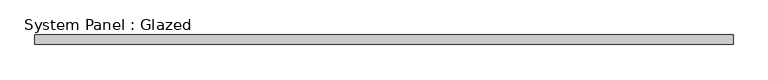
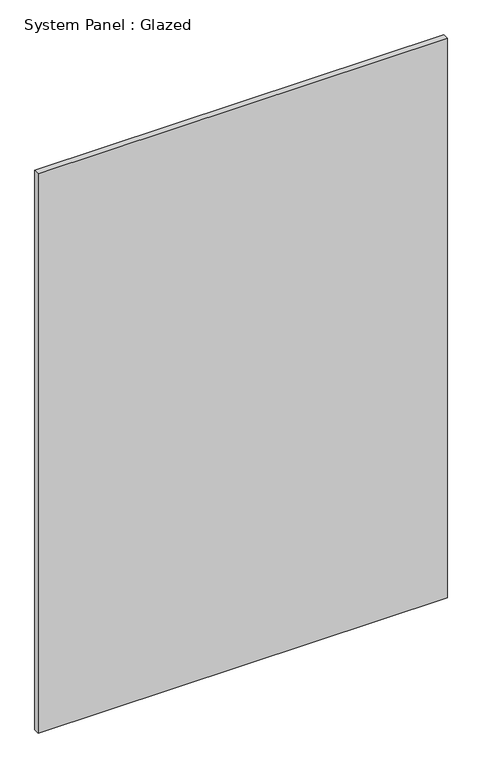
"""IFC4 building model written with IfcOpenShell, lengths in millimetres: plate geometry, System Panel : Glazed."""

from ifc_helpers import new_model, si_unit, origin, origin_with_axes, place, context, project, spatial, polyline, outline, extrude, source, transform, mapped, element, save


def system_panel_glazed_96f1d4d6(model_context):
    return source(origin(), model_context, "Body", "SweptSolid", [
        extrude(outline(polyline([(915.0, 24.5), (-915.0, 24.5), (-915.0, 49.5), (915.0, 49.5), (915.0, 24.5)])), origin_with_axes(), (0.0, 0.0, 1.0), 2643.2),
    ])


if __name__ == "__main__":
    model = new_model("IFC4")
    model_context = context("Model", 3, world=origin())
    ifc_project = project(units=[si_unit("LENGTHUNIT", "METRE", prefix="MILLI")], contexts=[model_context])
    site = spatial("IfcSite", under=ifc_project)
    building = spatial("IfcBuilding", under=site)
    placement = place(None, origin())
    system_panel_glazed_shape = system_panel_glazed_96f1d4d6(model_context)
    element("IfcPlate", 1, ObjectType="System Panel : Glazed", at=placement, inside=building, context=model_context, shape_type="MappedRepresentation", body=[
        mapped(system_panel_glazed_shape, transform((0.0, 0.0, 0.0), x_axis=(1.0, 0.0, 0.0), y_axis=(0.0, 1.0, 0.0), z_axis=(0.0, 0.0, 1.0))),
    ])
    save(model, "model.ifc")

# Revit data of these elements
# Type "System Panel : Glazed"
#   Construction Type Id = "GSP4R"
#   Analytic Construction = "1/8 in Pilkington single glazing"
#   Visual Light Transmittance = 0.9
#   Solar Heat Gain Coefficient = 0.86
#   Heat Transfer Coefficient (U) = 6.7069 W/(m²·K)
# Element 1 (IfcPlate, "System Panel : Glazed")
#   Materials on its faces: "Glass"
# Materials
#   "Glass": class "Glass", colour RGB 0 128 192, transparency 0.9, Description = "Soda Lime Glass", Cost = 0
